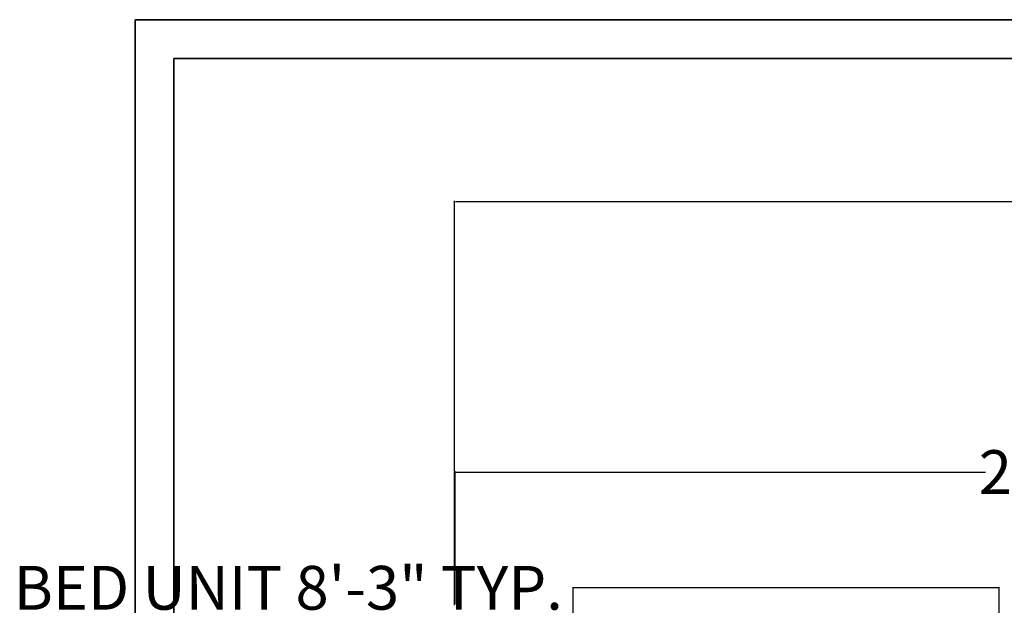
# Model space of a CAD drawing. Units: inches. Extents: x 1077 to 2505, y 1892 to 2728.
# Tile 13 of 26: x 1077 to 1306, y 2586 to 2722. Entities that reach past the tile are written whole.
import ezdxf

# ---------------------------------------------------------------- set-up
doc = ezdxf.new("R2010")
doc.units = ezdxf.units.IN
doc.linetypes.add('ACAD_ISO02W100', pattern=[15, 12, -3])
doc.layers.get('Defpoints').update_dxf_attribs({"color": 220, "linetype": 'ACAD_ISO02W100'})
doc.layers.add('A-ANNO-DIMS', color=2, linetype='Continuous', lineweight=18)
doc.layers.add('A-ANNO-TTLB', color=7, linetype='Continuous', lineweight=35)
doc.layers.add('A-FLOR-PATT', color=254, linetype='Continuous', lineweight=9, true_color=0xd7ebd2)
doc.styles.get("Standard").update_dxf_attribs({"font": 'arial.ttf'})
doc.dimstyles.get("Standard").update_dxf_attribs({"dimtxt": 10.18, "dimasz": 0.18, "dimexe": 0.18, "dimexo": 0.0625, "dimgap": 0.09, "dimtad": 0, "dimtih": 1, "dimtoh": 1, "dimdec": 0, "dimzin": 0, "dimdsep": 46, "dimlunit": 3, "dimtxsty": 'Standard', "dimcen": 0.09, "dimadec": 0, "dimazin": 0, "dimtfac": 1, "dimtdec": 0, "dimtofl": 0, "dimtmove": 0, "dimatfit": 3, "dimfxl": 1, "dimtolj": 1, "dimtzin": 0, "dimarcsym": 0})

# ---------------------------------------------------------------- blocks, each defined once
blk = doc.blocks.new('*D13')
at = {"layer": 'A-ANNO-DIMS', "color": 0, "lineweight": -2, "transparency": 16777216}
for p, q in [((1178.64, 2586.44), (1178.64, 2617.31)), ((1178.82, 2617.13), (1301.91, 2617.13)), ((1460.32, 2617.13), (1337.23, 2617.13)), ((1460.5, 2586.44), (1460.5, 2617.31))]:
    blk.add_line(p, q, dxfattribs=at)
at = {"layer": 'A-ANNO-DIMS', "color": 0, "transparency": 16777216}
for points in [[(1178.82, 2617.16), (1178.82, 2617.1), (1178.64, 2617.13)], [(1460.32, 2617.16), (1460.32, 2617.1), (1460.5, 2617.13)]]:
    blk.add_solid(points, dxfattribs=at)
at = {"layer": 'Defpoints', "color": 0, "transparency": 16777216}
for p in [(1460.5, 2617.13), (1178.64, 2586.38), (1460.5, 2586.38)]:
    blk.add_point(p, dxfattribs=at)
at = {"layer": 'A-ANNO-DIMS', "color": 0, "transparency": 16777216, "insert": (1319.57, 2617.13), "char_height": 10.18, "attachment_point": 5}
blk.add_mtext('\\A1;23\'-6"', dxfattribs=at)
blk = doc.blocks.new('SHEET-FRAME-RESIDENTIAL')
for points in [[(0, 830.04), (543.52, 830.04), (543.52, 0), (0, 0)], [(9, 821.04), (534.52, 821.04), (534.52, 9), (9, 9)]]:
    blk.add_lwpolyline(points, close=True)
blk = doc.blocks.new('*D32')
at = {"layer": 'A-ANNO-DIMS', "color": 0, "lineweight": -2, "transparency": 16777216}
for p, q in [((1206.09, 2590.23), (1205.91, 2590.23)), ((1206.09, 2575.45), (1206.09, 2590.41)), ((1304.91, 2590.23), (1206.27, 2590.23)), ((1305.09, 2575.45), (1305.09, 2590.41))]:
    blk.add_line(p, q, dxfattribs=at)
at = {"layer": 'A-ANNO-DIMS', "color": 0, "transparency": 16777216}
for points in [[(1206.27, 2590.26), (1206.27, 2590.2), (1206.09, 2590.23)], [(1304.91, 2590.26), (1304.91, 2590.2), (1305.09, 2590.23)]]:
    blk.add_solid(points, dxfattribs=at)
at = {"layer": 'Defpoints', "color": 0, "transparency": 16777216}
for p in [(1206.09, 2590.23), (1206.09, 2575.38), (1305.09, 2575.38)]:
    blk.add_point(p, dxfattribs=at)
at = {"layer": 'A-ANNO-DIMS', "color": 0, "transparency": 16777216, "insert": (1139.85, 2590.23), "char_height": 10.18, "attachment_point": 5}
blk.add_mtext('\\A1;BED UNIT 8\'-3" TYP.', dxfattribs=at)
blk = doc.blocks.new('*D62')
at = {"layer": 'A-ANNO-DIMS', "color": 0, "lineweight": -2, "transparency": 16777216}
for p, q in [((1178.53, 2586.22), (1178.53, 2680.19)), ((1556.53, 2651.22), (1556.53, 2680.19)), ((1178.71, 2680.01), (1349.96, 2680.01)), ((1556.35, 2680.01), (1385.1, 2680.01))]:
    blk.add_line(p, q, dxfattribs=at)
at = {"layer": 'A-ANNO-DIMS', "color": 0, "transparency": 16777216}
for points in [[(1178.71, 2680.04), (1178.71, 2679.98), (1178.53, 2680.01)], [(1556.35, 2680.04), (1556.35, 2679.98), (1556.53, 2680.01)]]:
    blk.add_solid(points, dxfattribs=at)
at = {"layer": 'Defpoints', "color": 0, "transparency": 16777216}
for p in [(1556.53, 2680.01), (1556.53, 2651.16), (1178.53, 2586.16)]:
    blk.add_point(p, dxfattribs=at)
at = {"layer": 'A-ANNO-DIMS', "color": 0, "transparency": 16777216, "insert": (1367.53, 2680.01), "char_height": 10.18, "attachment_point": 5}
blk.add_mtext('\\A1;31\'-6"', dxfattribs=at)

msp = doc.modelspace()

# ---------------------------------------------------------------- hatches: boundary and pattern name
at = {"layer": 'A-FLOR-PATT', "transparency": 33554559}
h = msp.add_hatch(color=256, dxfattribs=at)
h.dxf.hatch_style = 1
h.paths.add_polyline_path([(1395.53, 2577.16), (1374.83, 2577.16), (1350.83, 2577.19), (1350.83, 2577.16), (1329.53, 2577.16), (1329.53, 2480.16), (1329.53, 2469.16), (1325.53, 2469.16), (1325.53, 2515.13), (1307.53, 2515.13), (1307.53, 2577.16), (1269.31, 2577.16), (1221.31, 2577.15), (1221.31, 2577.16), (1187.53, 2577.16), (1187.53, 2433.16), (1289.53, 2433.16), (1289.53, 2429.16), (1263.53, 2429.16), (1187.53, 2429.16), (1187.53, 2395.02), (1187.53, 2395.02), (1187.53, 2371.02), (1187.53, 2371.02), (1187.53, 2307.16), (1259.53, 2307.16), (1259.53, 2399.16), (1263.53, 2399.16), (1263.53, 2307.16), (1289.53, 2307.16), (1289.53, 2306.23), (1325.53, 2306.23), (1325.53, 2307.16), (1329.53, 2307.16), (1329.53, 2306.23), (1365.53, 2306.23), (1365.53, 2307.16), (1432.53, 2307.16), (1432.53, 2088.16), (1547.53, 2088.16), (1547.53, 2140.08), (1511.53, 2140.08), (1511.53, 2267.16), (1475.53, 2267.16), (1475.53, 2303.16), (1468.53, 2303.16), (1468.53, 2307.16), (1547.53, 2307.16), (1547.53, 2348.22), (1547.53, 2396.22), (1547.53, 2429.16), (1435.53, 2429.16), (1435.53, 2433.16), (1476.35, 2433.16), (1476.35, 2451.18), (1547.53, 2451.18), (1547.53, 2577.16), (1499.53, 2577.16), (1499.53, 2586.16), (1547.53, 2586.16), (1547.53, 2642.16), (1518.18, 2642.16), (1518.18, 2642.05), (1494.15, 2642.05), (1494.15, 2642.16), (1469.53, 2642.16), (1469.53, 2577.16), (1399.53, 2577.16), (1399.53, 2429.16), (1325.53, 2429.16), (1325.53, 2433.16), (1329.53, 2433.16), (1395.53, 2433.16), (1395.53, 2480.16), (1359.53, 2480.16), (1359.53, 2484.16), (1395.53, 2484.16)])
h.paths.add_polyline_path([(1357.65, 2482.07), (1355.65, 2482.07), (1355.65, 2481.07, 0.414214), (1356.65, 2480.07), (1344.65, 2480.07), (1344.65, 2477.06), (1343.27, 2477.06), (1343.27, 2480.07), (1330.65, 2480.07, -0.414214), (1329.65, 2481.07), (1329.65, 2484.07), (1331.65, 2484.07), (1331.65, 2510.07, -0.446908)], flags=16)
h.paths.add_polyline_path([(1305.09, 2559.18), (1288.89, 2559.18), (1288.89, 2575.38), (1305.09, 2575.38)], flags=16)
h.paths.add_polyline_path([(1304.19, 2560.08), (1289.79, 2560.08), (1289.79, 2574.48), (1304.19, 2574.48)], flags=0)
h.paths.add_polyline_path([(1287.99, 2500.68, -0.414214), (1287.09, 2499.78), (1265.14, 2499.78), (1224.09, 2499.78, -0.414214), (1223.19, 2500.68), (1223.19, 2557.16), (1223.19, 2571.74), (1223.19, 2575.38), (1287.99, 2575.38), (1287.99, 2571.74), (1287.09, 2571.74, -0.414214), (1287.99, 2570.84)], flags=16)
h.paths.add_polyline_path([(1292.98, 2569.05, -1), (1300.92, 2569.05, -1)], flags=0)
h.paths.add_polyline_path([(1293.32, 2569.05, -1), (1300.58, 2569.05, -1)], flags=0)
h.paths.add_polyline_path([(1322.8, 2462.21), (1322.8, 2431.71), (1323.05, 2430.71), (1323.05, 2431.71), (1321.8, 2431.71), (1321.8, 2462.19, 0.404641), (1292.3, 2431.71), (1292.05, 2430.71, -0.414214), (1291.55, 2430.21), (1291.05, 2430.21), (1291.05, 2429.71, -0.414214), (1290.55, 2429.21), (1289.55, 2429.21), (1289.55, 2434.21), (1290.55, 2434.21, -0.414214), (1291.05, 2433.71), (1291.05, 2433.21), (1291.55, 2433.21, -0.414214), (1292.05, 2432.71), (1292.3, 2431.71, -0.414214)], flags=16)
h.paths.add_polyline_path([(1287.82, 2548.28, 0.292232), (1279.17, 2536.8, 0.052719), (1223.93, 2548.28), (1223.28, 2548.28), (1223.28, 2557.16), (1223.93, 2557.16), (1245.42, 2557.16, -0.117785), (1245.77, 2557.93, -0.059418), (1254.87, 2567.02, -0.379859), (1257.28, 2566.88, -0.02509), (1261.41, 2563.32, -0.025935), (1265.65, 2567.02, -0.379859), (1268.06, 2566.88, -0.061767), (1277.52, 2557.43, -0.069393), (1277.82, 2557.16), (1287.82, 2557.16)], flags=0)
h.paths.add_polyline_path([(1263.47, 2548.28), (1260.56, 2548.28, -0.015371), (1258.01, 2546.13, -0.429576), (1255.37, 2546.06, -0.016036), (1252.69, 2548.28), (1223.28, 2548.28), (1223.28, 2554.42), (1246.78, 2554.42, 0.055344), (1255.37, 2546.06, 0.331768), (1257.52, 2545.74, 0.027343), (1262, 2549.64, 0.00919)], flags=0)
h.paths.add_polyline_path([(1295.56, 2568.34), (1296.87, 2569.09), (1296.87, 2570.6, 0.399698), (1295.39, 2569.05, 0.119004)], flags=0)
h.paths.add_polyline_path([(1295.21, 2569.05, -1), (1298.68, 2569.05, -1)], flags=0)
h.paths.add_polyline_path([(1296.95, 2568.96), (1297.03, 2569), (1297.03, 2569.09), (1296.99, 2569.11), (1296.91, 2568.98)], flags=0)
h.paths.add_polyline_path([(1402.28, 2462.19, -0.414214), (1432.78, 2431.69), (1433.03, 2432.69), (1432.78, 2431.69, 0.404641), (1403.28, 2462.17), (1403.28, 2431.69), (1402.03, 2431.69), (1402.03, 2430.69, -0.414214), (1401.53, 2430.19), (1401.03, 2430.19), (1401.03, 2429.69, -0.414214), (1400.53, 2429.19), (1399.53, 2429.19), (1399.53, 2434.19), (1400.53, 2434.19, -0.414214), (1401.03, 2433.69), (1401.03, 2433.19), (1401.53, 2433.19, -0.414214), (1402.03, 2432.69)], flags=16)
h.paths.add_polyline_path([(1470.16, 2535.21, -0.414214), (1471.06, 2536.11), (1527.54, 2536.11), (1542.12, 2536.11), (1545.76, 2536.11), (1545.76, 2471.31), (1542.12, 2471.31), (1542.12, 2472.21, -0.414214), (1541.22, 2471.31), (1471.06, 2471.31, -0.414214), (1470.16, 2472.21), (1470.16, 2494.16)], flags=16)
h.paths.add_polyline_path([(1483.07, 2536.11, 0.253465), (1480.11, 2526.15, 0.2538), (1470.15, 2523.19)], flags=16)
h.paths.add_polyline_path([(1223.19, 2512.69, 0.253465), (1233.14, 2509.74, 0.2538), (1236.1, 2499.77)], flags=16)
h.paths.add_polyline_path([(1469.77, 2578.72), (1469.77, 2581.72), (1471.77, 2581.72), (1471.77, 2607.72, -0.01951), (1473.77, 2607.68), (1473.77, 2579.72), (1473.77, 2578.72, -0.414214), (1472.77, 2577.72), (1470.77, 2577.72, -0.414214)], flags=16)
h.paths.add_polyline_path([(1382.46, 2398.13), (1395.04, 2398.13), (1395.04, 2399.74), (1382.46, 2399.74)], flags=16)
h.paths.add_polyline_path([(1379.94, 2397.18), (1379.94, 2389.82), (1380.5, 2389.82), (1380.5, 2396.05, -0.41429), (1381.06, 2396.61), (1396.47, 2396.61, -0.414213), (1397.03, 2396.05), (1397.03, 2389.82), (1397.59, 2389.82), (1397.59, 2397.18)], flags=16)
h.paths.add_polyline_path([(1263.37, 2428.14), (1263.37, 2426.14, -0.414214), (1262.37, 2425.14), (1261.37, 2425.14), (1233.41, 2425.14, 0.400854), (1259.37, 2401.04), (1259.37, 2401.14), (1261.37, 2401.14, -0.446908), (1233.37, 2427.14), (1259.37, 2427.14), (1259.37, 2429.14), (1262.37, 2429.14, -0.414214)], flags=16)
h.paths.add_polyline_path([(1404.79, 2398.13), (1417.37, 2398.13), (1417.37, 2399.74), (1404.79, 2399.74)], flags=16)
h.paths.add_polyline_path([(1402.27, 2397.18), (1404.79, 2398.13), (1417.37, 2398.13), (1419.92, 2397.18)], flags=16)
h.paths.add_polyline_path([(1432.26, 2383.16), (1432.26, 2370.59), (1433.87, 2370.59), (1433.87, 2383.16)], flags=16)
h.paths.add_polyline_path([(1431.3, 2385.69), (1423.84, 2385.69), (1423.84, 2385.13), (1430.18, 2385.13, -0.41429), (1430.74, 2384.57), (1430.74, 2369.16, -0.414237), (1430.18, 2368.6), (1423.84, 2368.6), (1423.84, 2368.03), (1431.3, 2368.03)], flags=16)
h.paths.add_polyline_path([(1417.37, 2351.16), (1417.37, 2349.54), (1418.9, 2349.54, 0.414236), (1419.92, 2350.56), (1419.92, 2352.11)], flags=16)
h.paths.add_polyline_path([(1395.04, 2351.16), (1395.04, 2349.54), (1396.58, 2349.54, 0.414235), (1397.59, 2350.56), (1397.59, 2352.11)], flags=16)
h.paths.add_polyline_path([(1366.7, 2370.05), (1365.09, 2370.05), (1365.09, 2368.52, 0.414235), (1366.11, 2367.5), (1367.66, 2367.5)], flags=16)
h.paths.add_polyline_path([(1419.36, 2359.47), (1419.36, 2353.24, -0.41419), (1418.8, 2352.68), (1403.39, 2352.68, -0.414137), (1402.83, 2353.24), (1402.83, 2359.47), (1397.03, 2359.47), (1397.03, 2353.24, -0.414189), (1396.47, 2352.68), (1381.06, 2352.68, -0.414137), (1380.5, 2353.24), (1380.5, 2359.47)], flags=16)
h.paths.add_polyline_path([(1222.29, 2559.18), (1206.09, 2559.18), (1206.09, 2575.38), (1222.29, 2575.38)], flags=16)
h.paths.add_polyline_path([(1221.39, 2560.08), (1206.99, 2560.08), (1206.99, 2574.48), (1221.39, 2574.48)], flags=0)
h.paths.add_polyline_path([(1482, 2577.72), (1482, 2580.73), (1483.38, 2580.73), (1483.38, 2577.72), (1484.77, 2577.72), (1484.77, 2574.72), (1483.38, 2574.72), (1483.38, 2577.72)], flags=16)
h.paths.add_polyline_path([(1266.37, 2415.53), (1266.37, 2414.14), (1263.37, 2414.14), (1263.37, 2415.53), (1260.36, 2415.53), (1260.36, 2416.91), (1263.37, 2416.91), (1263.37, 2415.53)], flags=16)
h.paths.add_polyline_path([(1210.26, 2569.05, -1), (1218.19, 2569.05, -1)], flags=0)
h.paths.add_polyline_path([(1210.6, 2569.05, -1), (1217.85, 2569.05, -1)], flags=0)
h.paths.add_polyline_path([(1212.84, 2568.34), (1214.15, 2569.09), (1214.15, 2570.6, 0.399698), (1212.67, 2569.05, 0.119004)], flags=0)
h.paths.add_polyline_path([(1212.49, 2569.05, -1), (1215.96, 2569.05, -1)], flags=0)
h.paths.add_polyline_path([(1214.23, 2568.96), (1214.3, 2568.91), (1214.3, 2569)], flags=0)
h.paths.add_polyline_path([(1507.18, 2480.12, 0.052719), (1518.66, 2535.36), (1518.66, 2536.01), (1527.54, 2536.01), (1527.54, 2535.36), (1527.54, 2513.88, -0.117785), (1528.31, 2513.53, -0.059418), (1537.4, 2504.43, -0.379859), (1537.26, 2502.01, -0.02509), (1533.7, 2497.89, -0.025935), (1537.4, 2493.64, -0.379859), (1537.26, 2491.23, -0.061767), (1527.8, 2481.77, -0.069393), (1527.54, 2481.47), (1527.54, 2471.47), (1518.66, 2471.47, 0.292232)], flags=0)
h.paths.add_polyline_path([(1516.43, 2503.92, -0.016036), (1518.66, 2506.6), (1518.66, 2536.01), (1524.8, 2536.01), (1524.8, 2512.51, 0.055344), (1516.43, 2503.92, 0.331768), (1516.12, 2501.77, 0.027343), (1520.01, 2497.29, 0.00919), (1518.66, 2495.82), (1518.66, 2498.73, -0.015371), (1516.5, 2501.28, -0.429576)], flags=0)
h.paths.add_polyline_path([(1499.63, 2625.5, -0.171636), (1502.82, 2631.01), (1502.82, 2633.37), (1498.68, 2633.37, -0.414214), (1497.7, 2634.36), (1497.7, 2640.66, -0.414214), (1498.68, 2641.64), (1514.82, 2641.64, -0.414214), (1515.81, 2640.66), (1515.81, 2634.36, -0.414214), (1514.82, 2633.37), (1510.69, 2633.37), (1510.69, 2631.01, -0.171636), (1513.88, 2625.5, -0.258205), (1509.31, 2614.47), (1504.19, 2614.47, -0.258205)], flags=16)
h.paths.add_polyline_path([(1501.2, 2625.5, -0.171636), (1504.39, 2631.01), (1509.12, 2631.01, -0.171636), (1512.3, 2625.5, -0.210384), (1509.35, 2616.02), (1504.16, 2616.02, -0.210384)], flags=0)
h.paths.add_polyline_path([(1529.56, 2537.01), (1529.56, 2553.21), (1545.76, 2553.21), (1545.76, 2537.01)], flags=16)
h.paths.add_polyline_path([(1530.46, 2537.91), (1530.46, 2552.31), (1544.86, 2552.31), (1544.86, 2537.91)], flags=0)
h.paths.add_polyline_path([(1535.45, 2545.07, -1), (1543.39, 2545.07, -1)], flags=0)
h.paths.add_polyline_path([(1535.8, 2545.07, -1), (1543.05, 2545.07, -1)], flags=0)
h.paths.add_polyline_path([(1529.56, 2470.41), (1545.76, 2470.41), (1545.76, 2454.21), (1529.56, 2454.21)], flags=16)
h.paths.add_polyline_path([(1541.16, 2544.99), (1540.98, 2544.99, -0.544606), (1538.71, 2543.68), (1538.62, 2543.53, 0.547962)], flags=0)
h.paths.add_polyline_path([(1530.46, 2469.51), (1544.86, 2469.51), (1544.86, 2455.11), (1530.46, 2455.11)], flags=0)
h.paths.add_polyline_path([(1539.47, 2545.14), (1539.42, 2545.22), (1539.38, 2545.14)], flags=0)
h.paths.add_polyline_path([(1543.39, 2462.34, -1), (1535.45, 2462.34, -1)], flags=0)
h.paths.add_polyline_path([(1543.05, 2462.34, -1), (1535.8, 2462.34, -1)], flags=0)
h.paths.add_polyline_path([(1541.16, 2462.27), (1540.98, 2462.27, -0.544606), (1538.71, 2460.96), (1538.62, 2460.8, 0.547962)], flags=0)
h.paths.add_polyline_path([(1539.47, 2462.42), (1539.42, 2462.5), (1539.38, 2462.42)], flags=0)
h.paths.add_polyline_path([(1435.32, 2335.25, -0.414214), (1465.82, 2304.75), (1466.07, 2305.75), (1465.82, 2304.75, 0.404641), (1436.32, 2335.23), (1436.32, 2304.75), (1435.07, 2304.75), (1435.07, 2303.75, -0.414214), (1434.57, 2303.25), (1434.07, 2303.25), (1434.07, 2302.75, -0.414214), (1433.57, 2302.25), (1432.57, 2302.25), (1432.57, 2307.25), (1433.57, 2307.25, -0.414214), (1434.07, 2306.75), (1434.07, 2306.25), (1434.57, 2306.25, -0.414214), (1435.07, 2305.75)], flags=16)
h.paths.add_polyline_path([(1532.13, 2635.71), (1535.43, 2635.71), (1535.43, 2635.89), (1532.13, 2635.89)], flags=16)
edge = h.paths.add_edge_path(flags=16)
edge.add_arc((1535.98, 2632.67), 0.183, 270, 360)
edge.add_line((1536.17, 2632.67), (1536.17, 2639.82))
edge.add_line((1536.17, 2639.82), (1538.29, 2639.82))
edge.add_line((1538.29, 2639.82), (1538.29, 2641.82))
edge.add_line((1538.29, 2641.82), (1533.25, 2641.82))
edge.add_line((1533.25, 2641.82), (1533.25, 2639.82))
edge.add_line((1533.25, 2639.82), (1534.87, 2639.82))
edge.add_line((1534.87, 2639.82), (1534.87, 2639))
edge.add_line((1534.87, 2639), (1533.7, 2639))
edge.add_line((1533.7, 2639), (1533.7, 2639.82))
edge.add_line((1533.7, 2639.82), (1533.25, 2639.82))
edge.add_line((1533.25, 2639.82), (1533.25, 2641.82))
edge.add_line((1533.25, 2641.82), (1538.29, 2641.82))
edge.add_line((1538.29, 2641.82), (1538.29, 2641.34))
edge.add_line((1538.29, 2641.34), (1540.64, 2641.58))
edge.add_line((1540.64, 2641.58), (1540.64, 2641.82))
edge.add_line((1540.64, 2641.82), (1541.5, 2641.82))
edge.add_line((1541.5, 2641.82), (1541.5, 2641.25))
edge.add_line((1541.5, 2641.25), (1541.31, 2639.79))
edge.add_ellipse((1541.09, 2638.95), major_axis=(-1.08, 0), ratio=0.790849, start_angle=180, end_angle=255.2976, ccw=False)
edge.add_line((1542.17, 2638.95), (1542.17, 2638.38))
edge.add_ellipse((1541.09, 2638.38), major_axis=(-1.08, 0), ratio=0.790849, start_angle=0, end_angle=180, ccw=False)
edge.add_line((1540, 2638.38), (1540.01, 2638.87))
edge.add_ellipse((1541.09, 2638.95), major_axis=(-1.08, 0), ratio=0.790849, start_angle=284.7024, end_angle=364.0401, ccw=False)
edge.add_line((1540.78, 2639.75), (1540.78, 2641.25))
edge.add_line((1540.78, 2641.25), (1540.64, 2641.25))
edge.add_line((1540.64, 2641.25), (1538.29, 2641.01))
edge.add_line((1538.29, 2641.01), (1538.29, 2639.82))
edge.add_line((1538.29, 2639.82), (1536.17, 2639.82))
edge.add_line((1536.17, 2639.82), (1536.17, 2632.48))
edge.add_line((1536.17, 2632.48), (1535.98, 2632.48))
h.paths.add_polyline_path([(1496.32, 2250.34, -0.292371), (1498.9, 2247.83, -0.085148), (1501.21, 2208.85, -0.01331), (1500.27, 2098.5, -0.379287), (1497.22, 2095.28, -0.0502), (1441.54, 2095.28, -0.379287), (1438.5, 2098.5, -0.01331), (1437.56, 2208.85, -0.086132), (1439.96, 2248.26, -0.295116), (1442.59, 2250.78, -0.114238)], flags=16)
h.paths.add_polyline_path([(1495.16, 2205.84, -0.355389), (1496.7, 2202.1), (1492.94, 2189.65, -0.398275), (1489.12, 2187.47, 0.113332), (1449.64, 2187.47, -0.398275), (1445.82, 2189.65), (1442.06, 2202.1, -0.355394), (1443.6, 2205.84, -0.265725)], flags=0)
h.paths.add_polyline_path([(1440.37, 2195.72), (1445.94, 2181.67), (1445.94, 2160.63), (1440.84, 2157.26)], flags=0)
h.paths.add_polyline_path([(1498.46, 2195.72), (1497.99, 2157.26), (1492.88, 2160.63), (1492.88, 2181.67)], flags=0)
h.paths.add_polyline_path([(1445.94, 2158.37), (1445.94, 2137.12), (1441.12, 2122.56), (1440.87, 2155.03)], flags=0)
h.paths.add_polyline_path([(1492.88, 2158.37), (1497.96, 2155.03), (1497.71, 2122.56), (1492.88, 2137.12)], flags=0)
h.paths.add_polyline_path([(1489.88, 2130.4), (1494.39, 2107.67, -0.090102), (1444.44, 2107.65), (1448.95, 2130.39, 0.036636)], flags=0)
h.paths.add_polyline_path([(1447.54, 2159.34), (1497.44, 2159.34), (1497.44, 2177.89), (1447.54, 2177.89)], flags=8)
h.paths.add_polyline_path([(1196.44, 2354.84), (1246.65, 2354.84), (1246.65, 2388.43), (1196.44, 2388.43)], flags=24)
h.paths.add_polyline_path([(1296.09, 2360.25), (1353.81, 2360.25), (1353.81, 2393.84), (1296.09, 2393.84)], flags=24)
h.paths.add_polyline_path([(1400.72, 2471.85), (1470.63, 2471.85), (1470.63, 2505.44), (1400.72, 2505.44)], flags=24)
h.paths.add_polyline_path([(1324.78, 2448.48), (1394.95, 2448.48), (1394.95, 2467.02), (1324.78, 2467.02)], flags=24)
h.paths.add_polyline_path([(1335.08, 2531.43), (1389.67, 2531.43), (1389.67, 2565.02), (1335.08, 2565.02)], flags=24)
h.paths.add_polyline_path([(1225.76, 2460), (1295.67, 2460), (1295.67, 2493.58), (1225.76, 2493.58)], flags=24)

# ---------------------------------------------------------------- block references
at = {"layer": 'A-ANNO-TTLB'}
msp.add_blockref('SHEET-FRAME-RESIDENTIAL', (1104.25, 1892.27), dxfattribs=at)

# ---------------------------------------------------------------- dimensions: what is measured, and where the dimension line sits
at = {"layer": 'A-ANNO-DIMS'}
for base, p1, p2, override, picture, middle in [((1556.53, 2680.01), (1178.53, 2586.16), (1556.53, 2651.16), {"dimdec": 1, "dimlfac": 1, "dimrnd": 0, "dimzin": 1, "dimdsep": 46, "dimlunit": 4, "dimfrac": 2}, '*D62', (1367.53, 2680.01)), ((1460.5, 2617.13), (1178.64, 2586.38), (1460.5, 2586.38), {"dimclrd": 0, "dimclre": 0, "dimclrt": 0}, '*D13', (1319.57, 2617.13))]:
    dim = msp.add_linear_dim(base=base, p1=p1, p2=p2, dimstyle='Standard', override=override, dxfattribs=at)
    dim.commit()
    dim.dimension.update_dxf_attribs({"geometry": picture, "text_midpoint": middle})
dim = msp.add_linear_dim(base=(1206.09, 2590.23), p1=(1305.09, 2575.38), p2=(1206.09, 2575.38), angle=180, text='BED UNIT <> TYP.', dimstyle='Standard', override={"dimdec": 1, "dimlfac": 1, "dimrnd": 0, "dimzin": 1, "dimdsep": 46, "dimlunit": 4, "dimfrac": 2}, dxfattribs=at)
dim.commit()
dim.dimension.update_dxf_attribs({"geometry": '*D32', "text_midpoint": (1139.85, 2590.23)})

doc.saveas('drawing.dxf')
